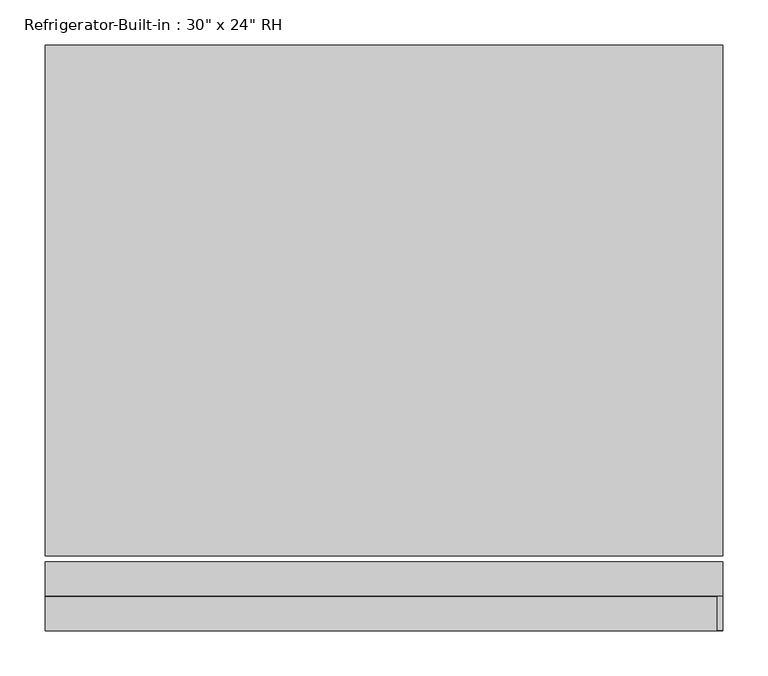
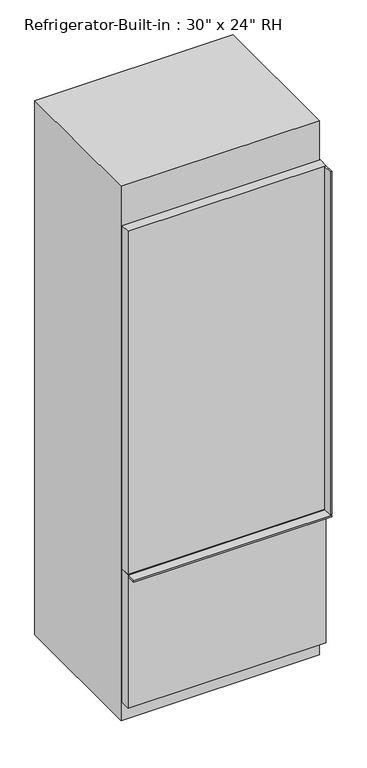
"""IFC4 building model written with IfcOpenShell, lengths in millimetres: proxy geometry."""

from ifc_helpers import new_model, si_unit, frame, origin, origin_with_axes, place, context, project, spatial, polyline, outline, extrude, source, transform, mapped, element, save


def proxy_e6cf46b9(model_context):
    return source(origin(), model_context, "Body", "SweptSolid", [
        extrude(outline(polyline([(374.65, 290.1239715), (374.65, -275.0260285), (-374.65, -275.0260285), (-374.65, 290.1239715), (374.65, 290.1239715)])), origin_with_axes(), (0.0, 0.0, 1.0), 2133.6),
        extrude(outline(polyline([(374.65, -281.3760285), (374.65, -319.4760285), (-374.65, -319.4760285), (-374.65, -281.3760285), (374.65, -281.3760285)])), frame((0.0, 0.0, 611.1875), z_axis=(0.0, 0.0, 1.0), x_axis=(1.0, 0.0, 0.0)), (0.0, 0.0, 1.0), 1370.0125),
        extrude(outline(polyline([(374.65, -281.3760285), (374.65, -319.4760285), (-374.65, -319.4760285), (-374.65, -281.3760285), (374.65, -281.3760285)])), frame((0.0, 0.0, 76.2), z_axis=(0.0, 0.0, 1.0), x_axis=(1.0, 0.0, 0.0)), (0.0, 0.0, 1.0), 531.8125),
        extrude(outline(polyline([(374.65, -319.4760285), (374.65, -357.5760285), (-374.65, -357.5760285), (-374.65, -319.4760285), (374.65, -319.4760285)])), frame((0.0, 0.0, 601.6625), z_axis=(0.0, 0.0, 1.0), x_axis=(1.0, 0.0, 0.0)), (0.0, 0.0, 1.0), 6.35),
        extrude(outline(polyline([(368.3, -319.4760285), (374.65, -319.4760285), (374.65, -357.5760285), (368.3, -357.5760285), (368.3, -319.4760285)])), frame((0.0, 0.0, 611.1875), z_axis=(0.0, 0.0, 1.0), x_axis=(1.0, 0.0, 0.0)), (0.0, 0.0, 1.0), 1370.0125),
    ])


if __name__ == "__main__":
    model = new_model("IFC4")
    model_context = context("Model", 3, world=origin())
    ifc_project = project(units=[si_unit("LENGTHUNIT", "METRE", prefix="MILLI")], contexts=[model_context])
    site = spatial("IfcSite", under=ifc_project)
    building = spatial("IfcBuilding", under=site)
    placement = place(None, origin())
    proxy_shape = proxy_e6cf46b9(model_context)
    element("IfcBuildingElementProxy", 1, Name="Refrigerator-Built-in : 30\" x 24\" RH", ObjectType="Refrigerator-Built-in : 30\" x 24\" RH", at=placement, inside=building, context=model_context, shape_type="MappedRepresentation", body=[
        mapped(proxy_shape, transform((0.0, 0.0, 0.0), x_axis=(1.0, 0.0, 0.0), y_axis=(0.0, 1.0, 0.0), z_axis=(0.0, 0.0, 1.0))),
    ])
    save(model, "model.ifc")

# Revit data of these elements
# Type "Refrigerator-Built-in : 30\" x 24\" RH"
#   Assembly Code = "E1090400"
#   Depth = 2' - 0"
#   Handle = 2' - 5 1/2"
#   Height = 7' - 0"
#   Top Door Height = 5' - 0"
#   Width = 2' - 5 1/2"
#   Material = Metal - Paint Finish - Ivory,Glossy
#   Default Elevation = 0
# Element 1 (IfcBuildingElementProxy, "Refrigerator-Built-in : 30\" x 24\" RH")
#   Materials on its faces: "Metal - Paint Finish - Ivory,Glossy", "Metal - Chrome"
# Materials
#   "Metal - Paint Finish - Ivory,Glossy": colour RGB 247 247 239, transparency 0
#   "Metal - Chrome": colour RGB 57 57 57, transparency 0
